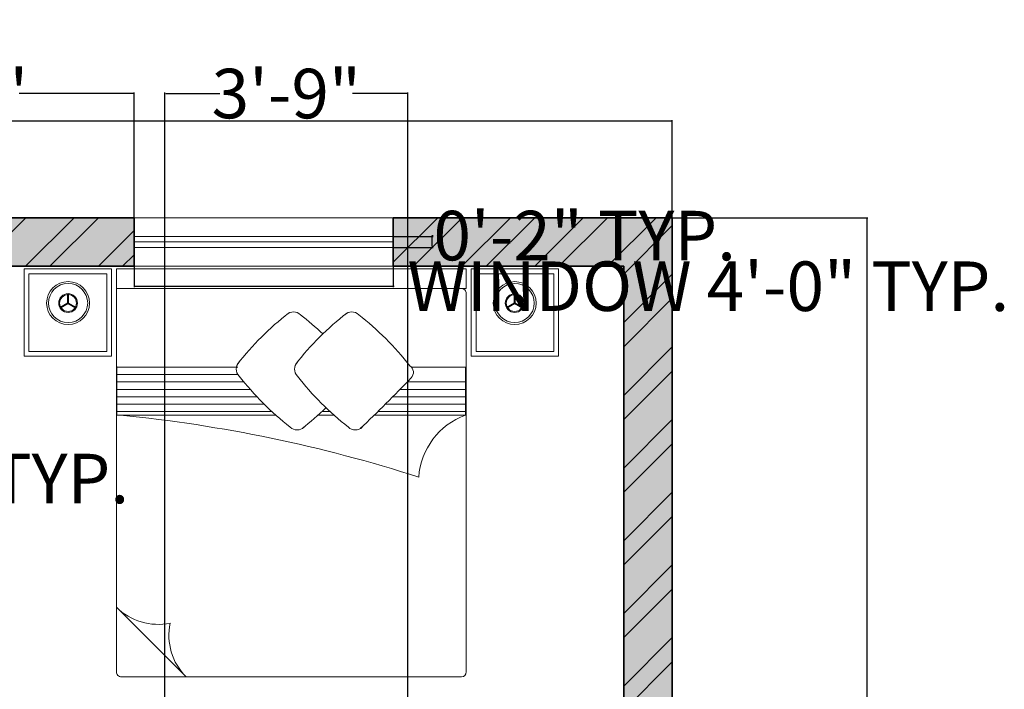
# Model space of a CAD drawing. Units: inches. Extents: x 1086 to 1540, y 3343 to 3848.
# Tile 8 of 8: x 1350 to 1532, y 3724 to 3848. Entities that reach past the tile are written whole.
import ezdxf

# ---------------------------------------------------------------- set-up
doc = ezdxf.new("R2010")
doc.units = ezdxf.units.IN
for name, color, linetype, lineweight in [('00 FURNITURE', 15, 'Continuous', 15), ('A-ANNO-DIMS', 2, 'Continuous', 13), ('A-WALL-PATT', 252, 'Continuous', 9), ('WALL', 7, 'Continuous', 35), ('WINDOW', 160, 'Continuous', 15)]:
    doc.layers.add(name, color=color, linetype=linetype, lineweight=lineweight)
doc.styles.get("Standard").update_dxf_attribs({"font": 'arial.ttf'})
doc.dimstyles.get("Standard").update_dxf_attribs({"dimtxt": 9.18, "dimasz": 0.18, "dimexe": 0.18, "dimexo": 0.0625, "dimgap": 0.09, "dimtad": 0, "dimtih": 1, "dimtoh": 1, "dimdec": 1, "dimzin": 0, "dimdsep": 46, "dimlunit": 3, "dimtxsty": 'Standard', "dimcen": 0.09, "dimadec": 0, "dimazin": 0, "dimtfac": 1, "dimtdec": 1, "dimtofl": 0, "dimtmove": 0, "dimatfit": 3, "dimfxl": 1, "dimtolj": 1, "dimtzin": 0, "dimarcsym": 0})

# ---------------------------------------------------------------- blocks, each defined once
blk = doc.blocks.new('RGWTG')
at = {"layer": '00 FURNITURE'}
for p, q in [((578.23, 3473.51), (577.36, 3475.01)), ((578.36, 3473.58), (577.49, 3475.09)), ((578.23, 3473.58), (577.36, 3472.08)), ((578.36, 3473.51), (577.49, 3472)), ((578.29, 3473.62), (580.03, 3473.62)), ((578.29, 3473.47), (580.03, 3473.47)), ((521.93, 3464.58), (509.03, 3451.68)), ((509.03, 3422.63), (509.03, 3463.68)), ((509.93, 3464.58), (566.4, 3464.58)), ((557.53, 3463.84), (557.53, 3464.49)), ((557.53, 3464.49), (566.4, 3464.49)), ((558.2, 3464.49), (558.2, 3435.82)), ((559.57, 3464.49), (559.57, 3437.25)), ((560.94, 3464.49), (560.94, 3438.58)), ((562.3, 3464.49), (562.3, 3439.83)), ((563.67, 3464.49), (563.67, 3440.99)), ((565.04, 3464.49), (565.04, 3442.08)), ((566.4, 3464.58), (580.98, 3464.58)), ((566.4, 3464.49), (566.4, 3442.08)), ((566.4, 3464.49), (566.4, 3463.84)), ((580.98, 3464.58), (580.98, 3416.72)), ((558.2, 3426.48), (558.2, 3425.04)), ((509.03, 3400.68), (509.03, 3422.63)), ((558.2, 3416.13), (558.2, 3399.95)), ((580.98, 3416.72), (580.98, 3400.68)), ((559.57, 3414.75), (559.57, 3399.95)), ((560.94, 3413.39), (560.94, 3399.95)), ((562.3, 3412.04), (562.3, 3399.95)), ((563.67, 3410.72), (563.67, 3399.95)), ((580.08, 3399.78), (509.93, 3399.78)), ((557.53, 3399.95), (557.53, 3400.6)), ((566.4, 3399.95), (557.53, 3399.95)), ((566.4, 3400.6), (566.4, 3399.95)), ((578.23, 3390.78), (577.36, 3392.29)), ((578.36, 3390.86), (577.49, 3392.36)), ((578.23, 3390.86), (577.36, 3389.36)), ((578.36, 3390.78), (577.49, 3389.28)), ((578.29, 3390.9), (580.03, 3390.9)), ((578.29, 3390.74), (580.03, 3390.74))]:
    blk.add_line(p, q, dxfattribs=at)
for points in [[(568.43, 3465.48), (584.63, 3465.48), (584.63, 3481.68), (568.43, 3481.68)], [(569.33, 3466.38), (583.73, 3466.38), (583.73, 3480.78), (569.33, 3480.78)], [(580.98, 3399.78), (584.63, 3399.78), (584.63, 3464.58), (580.98, 3464.58)], [(568.43, 3398.88), (584.63, 3398.88), (584.63, 3382.68), (568.43, 3382.68)], [(569.33, 3397.98), (583.73, 3397.98), (583.73, 3383.58), (569.33, 3383.58)]]:
    blk.add_lwpolyline(points, close=True, dxfattribs=at)
for points in [[(566.52, 3464.49), (557.53, 3464.49), (557.53, 3435.08)], [(557.53, 3427.21), (557.53, 3424.3)], [(557.53, 3416.82), (557.53, 3399.95), (566.4, 3399.95), (566.4, 3409.94)]]:
    blk.add_lwpolyline(points, dxfattribs=at)
for centre, radius in [((578.29, 3473.54), 3.97), ((578.29, 3473.54), 3.63), ((578.29, 3473.54), 1.74), ((578.29, 3473.54), 1.56), ((578.29, 3390.82), 3.97), ((578.29, 3390.82), 3.63), ((578.29, 3390.82), 1.74), ((578.29, 3390.82), 1.56)]:
    blk.add_circle(centre, radius, dxfattribs=at)
for centre, radius, start, end in [((509.93, 3463.68), 0.9, 90, 180), ((529.65, 3456.88), 10.9, 135.0361, 191.9278), ((290.56, 3490.52), 268.3, 342.2214, 354.2925), ((516.73, 3443.97), 10.9, 78.0722, 134.9639), ((598.15, 3399.01), 54.32, 127.931, 142.069), ((566.05, 3440.57), 1.82, 45, 135), ((533.58, 3399.31), 54.32, 37.931, 52.069), ((556.59, 3431.11), 1.82, 135, 225), ((574.84, 3431.77), 1.82, 315, 45), ((598.15, 3388.23), 54.32, 127.931, 142.069), ((566.05, 3429.78), 1.82, 45, 135), ((533.58, 3388.53), 54.32, 37.931, 52.069), ((533.28, 3463.88), 54.32, 316.32, 322.069), ((597.87, 3463.6), 54.32, 217.931, 224.141), ((556.59, 3420.33), 1.82, 135, 225), ((574.84, 3420.99), 1.82, 315, 45), ((765.33, 3619.75), 290.45, 223.6069, 226.2326), ((533.28, 3453.1), 54.32, 307.931, 322.069), ((545.02, 3395.29), 13.35, 20.4224, 85.5825), ((565.44, 3411.05), 1.47, 225.9674, 326.8337), ((509.93, 3400.68), 0.9, 180, 270), ((580.08, 3400.68), 0.9, 270, 0)]:
    blk.add_arc(centre, radius, start, end, dxfattribs=at)
blk = doc.blocks.new('*D12')
at = {"layer": 'A-ANNO-DIMS', "color": 0, "lineweight": -2, "transparency": 16777216}
for p, q in [((1194.74, 3811.63), (1194.74, 3829.64)), ((1194.92, 3829.46), (1324.78, 3829.46)), ((1470.56, 3829.46), (1340.7, 3829.46)), ((1470.74, 3811.63), (1470.74, 3829.64))]:
    blk.add_line(p, q, dxfattribs=at)
at = {"layer": 'A-ANNO-DIMS', "color": 0, "transparency": 16777216}
for points in [[(1194.92, 3829.49), (1194.92, 3829.43), (1194.74, 3829.46)], [(1470.56, 3829.49), (1470.56, 3829.43), (1470.74, 3829.46)]]:
    blk.add_solid(points, dxfattribs=at)
at = {"layer": 'Defpoints', "color": 0, "transparency": 16777216}
for p in [(1470.74, 3829.46), (1194.74, 3811.57), (1470.74, 3811.57)]:
    blk.add_point(p, dxfattribs=at)
at = {"layer": 'A-ANNO-DIMS', "color": 0, "transparency": 16777216, "insert": (1332.74, 3829.46), "char_height": 9.18, "attachment_point": 5}
blk.add_mtext("\\A1;23'", dxfattribs=at)
blk = doc.blocks.new('*D13')
at = {"layer": 'A-ANNO-DIMS', "color": 0, "lineweight": -2, "transparency": 16777216}
for p, q in [((1470.8, 3811.57), (1506.93, 3811.57)), ((1506.75, 3811.39), (1506.75, 3600.35)), ((1506.75, 3379.75), (1506.75, 3590.79)), ((1470.8, 3379.57), (1506.93, 3379.57))]:
    blk.add_line(p, q, dxfattribs=at)
at = {"layer": 'A-ANNO-DIMS', "color": 0, "transparency": 16777216}
for points in [[(1506.72, 3811.39), (1506.78, 3811.39), (1506.75, 3811.57)], [(1506.72, 3379.75), (1506.78, 3379.75), (1506.75, 3379.57)]]:
    blk.add_solid(points, dxfattribs=at)
at = {"layer": 'Defpoints', "color": 0, "transparency": 16777216}
for p in [(1470.74, 3811.57), (1470.74, 3379.57), (1506.75, 3379.57)]:
    blk.add_point(p, dxfattribs=at)
at = {"layer": 'A-ANNO-DIMS', "color": 0, "transparency": 16777216, "insert": (1506.75, 3595.57), "char_height": 9.18, "attachment_point": 5}
blk.add_mtext("\\A1;36'", dxfattribs=at)
blk = doc.blocks.new('WIN-GLAZING-48IN')
for p, q in [((48, 1), (0, 1)), ((48, 0), (0, 0)), ((48, -1), (0, -1))]:
    blk.add_line(p, q)
blk = doc.blocks.new('*D22')
at = {"layer": 'A-ANNO-DIMS', "color": 0, "lineweight": -2, "transparency": 16777216}
for p, q in [((1316.51, 3801.03), (1331.48, 3801.03)), ((1331.3, 3800.85), (1331.3, 3768.07)), ((1331.3, 3725.61), (1331.3, 3758.39)), ((1316.51, 3725.43), (1331.48, 3725.43))]:
    blk.add_line(p, q, dxfattribs=at)
at = {"layer": 'A-ANNO-DIMS', "color": 0, "transparency": 16777216}
for points in [[(1331.27, 3800.85), (1331.33, 3800.85), (1331.3, 3801.03)], [(1331.27, 3725.61), (1331.33, 3725.61), (1331.3, 3725.43)]]:
    blk.add_solid(points, dxfattribs=at)
at = {"layer": 'Defpoints', "color": 0, "transparency": 16777216}
for p in [(1316.45, 3801.03), (1331.3, 3801.03), (1316.45, 3725.43)]:
    blk.add_point(p, dxfattribs=at)
at = {"layer": 'A-ANNO-DIMS', "color": 0, "transparency": 16777216, "insert": (1331.3, 3763.23), "char_height": 9.18, "attachment_point": 5}
blk.add_mtext('\\A1;6\'-3 1/2" TYP.', dxfattribs=at)
blk = doc.blocks.new('*D23')
at = {"layer": 'A-ANNO-DIMS', "color": 0, "lineweight": -2, "transparency": 16777216}
for p, q in [((1371.06, 3806.01), (1371.06, 3798.69)), ((1419.06, 3806.01), (1419.06, 3798.69)), ((1371.24, 3798.87), (1418.88, 3798.87)), ((1419.06, 3798.87), (1419.24, 3798.87))]:
    blk.add_line(p, q, dxfattribs=at)
at = {"layer": 'A-ANNO-DIMS', "color": 0, "transparency": 16777216}
for points in [[(1371.24, 3798.9), (1371.24, 3798.84), (1371.06, 3798.87)], [(1418.88, 3798.9), (1418.88, 3798.84), (1419.06, 3798.87)]]:
    blk.add_solid(points, dxfattribs=at)
at = {"layer": 'Defpoints', "color": 0, "transparency": 16777216}
for p in [(1371.06, 3806.07), (1419.06, 3806.07), (1419.06, 3798.87)]:
    blk.add_point(p, dxfattribs=at)
at = {"layer": 'A-ANNO-DIMS', "color": 0, "transparency": 16777216, "insert": (1477.41, 3798.87), "char_height": 9.18, "attachment_point": 5}
blk.add_mtext('\\A1;WINDOW 4\'-0" TYP.', dxfattribs=at)
blk = doc.blocks.new('*D24')
at = {"layer": 'A-ANNO-DIMS', "color": 0, "lineweight": -2, "transparency": 16777216}
for p, q in [((1419.12, 3808.07), (1426.44, 3808.07)), ((1426.26, 3808.07), (1426.26, 3808.25)), ((1426.26, 3808.25), (1426.44, 3808.25)), ((1426.26, 3806.25), (1426.26, 3807.89)), ((1419.12, 3806.07), (1426.44, 3806.07))]:
    blk.add_line(p, q, dxfattribs=at)
at = {"layer": 'A-ANNO-DIMS', "color": 0, "transparency": 16777216}
for points in [[(1426.23, 3807.89), (1426.29, 3807.89), (1426.26, 3808.07)], [(1426.23, 3806.25), (1426.29, 3806.25), (1426.26, 3806.07)]]:
    blk.add_solid(points, dxfattribs=at)
at = {"layer": 'Defpoints', "color": 0, "transparency": 16777216}
for p in [(1419.06, 3808.07), (1426.26, 3808.07), (1419.06, 3806.07)]:
    blk.add_point(p, dxfattribs=at)
at = {"layer": 'A-ANNO-DIMS', "color": 0, "transparency": 16777216, "insert": (1454.51, 3808.25), "char_height": 9.18, "attachment_point": 5}
blk.add_mtext('\\A1;0\'-2" TYP.', dxfattribs=at)
blk = doc.blocks.new('*D48')
at = {"layer": 'A-ANNO-DIMS', "color": 0, "lineweight": -2, "transparency": 16777216}
for p, q in [((1282.55, 3811.63), (1282.55, 3834.75)), ((1282.73, 3834.57), (1303.86, 3834.57)), ((1370.88, 3834.57), (1349.75, 3834.57)), ((1371.06, 3811.63), (1371.06, 3834.75))]:
    blk.add_line(p, q, dxfattribs=at)
at = {"layer": 'A-ANNO-DIMS', "color": 0, "transparency": 16777216}
for points in [[(1282.73, 3834.6), (1282.73, 3834.54), (1282.55, 3834.57)], [(1370.88, 3834.6), (1370.88, 3834.54), (1371.06, 3834.57)]]:
    blk.add_solid(points, dxfattribs=at)
at = {"layer": 'Defpoints', "color": 0, "transparency": 16777216}
for p in [(1371.06, 3834.57), (1282.55, 3811.57), (1371.06, 3811.57)]:
    blk.add_point(p, dxfattribs=at)
at = {"layer": 'A-ANNO-DIMS', "color": 0, "transparency": 16777216, "insert": (1326.8, 3834.57), "char_height": 9.18, "attachment_point": 5}
blk.add_mtext('\\A1;7\'-4 1/2"', dxfattribs=at)
blk = doc.blocks.new('*D70')
at = {"layer": 'A-ANNO-DIMS', "color": 0, "lineweight": -2, "transparency": 16777216}
for p, q in [((1376.74, 3634.63), (1376.74, 3834.75)), ((1376.92, 3834.57), (1386.95, 3834.57)), ((1421.56, 3834.57), (1411.53, 3834.57)), ((1421.74, 3634.63), (1421.74, 3834.75))]:
    blk.add_line(p, q, dxfattribs=at)
at = {"layer": 'A-ANNO-DIMS', "color": 0, "transparency": 16777216}
for points in [[(1376.92, 3834.6), (1376.92, 3834.54), (1376.74, 3834.57)], [(1421.56, 3834.6), (1421.56, 3834.54), (1421.74, 3834.57)]]:
    blk.add_solid(points, dxfattribs=at)
at = {"layer": 'Defpoints', "color": 0, "transparency": 16777216}
for p in [(1421.74, 3834.57), (1376.74, 3634.57), (1421.74, 3634.57)]:
    blk.add_point(p, dxfattribs=at)
at = {"layer": 'A-ANNO-DIMS', "color": 0, "transparency": 16777216, "insert": (1399.24, 3834.57), "char_height": 9.18, "attachment_point": 5}
blk.add_mtext('\\A1;3\'-9"', dxfattribs=at)

msp = doc.modelspace()

# ---------------------------------------------------------------- hatches: boundary and pattern name
at = {"layer": 'A-WALL-PATT'}
h = msp.add_hatch(dxfattribs=at)
h.set_pattern_fill('ANSI32', color=256)
h.paths.add_polyline_path([(1234.55, 3811.57), (1234.55, 3811.57), (1194.74, 3811.57), (1194.74, 3622.57), (1203.74, 3622.57), (1203.74, 3634.57), (1218.33, 3634.57), (1218.33, 3638.57), (1203.74, 3638.57), (1203.74, 3802.57), (1234.55, 3802.57)])
h.paths.add_polyline_path([(1371.06, 3811.57), (1371.06, 3811.57), (1282.55, 3811.57), (1282.55, 3802.57), (1331.74, 3802.57), (1331.74, 3634.57), (1335.74, 3634.57), (1335.74, 3639.57), (1335.74, 3802.57), (1371.06, 3802.57)])
h.paths.add_polyline_path([(1470.74, 3811.57), (1419.06, 3811.57), (1419.06, 3802.57), (1461.74, 3802.57), (1461.74, 3638.57), (1461.74, 3548.57), (1425.74, 3548.57), (1425.74, 3582.21), (1421.74, 3582.21), (1421.74, 3548.57), (1376.74, 3548.57), (1376.74, 3602.57), (1373.71, 3602.57), (1372.74, 3602.57), (1372.74, 3544.57), (1461.74, 3544.57), (1461.74, 3379.57), (1470.74, 3379.57)])
h.paths.add_polyline_path([(1203.74, 3582.57), (1295.74, 3582.57), (1295.74, 3586.57), (1203.74, 3586.57), (1203.74, 3598.57), (1194.74, 3598.57), (1194.74, 3379.57), (1326.74, 3379.57), (1326.74, 3388.57), (1322.74, 3388.57), (1203.74, 3388.57), (1203.74, 3451.57), (1234.74, 3451.57), (1234.74, 3455.57), (1203.74, 3455.57), (1203.74, 3479.57), (1203.74, 3544.57), (1227.74, 3544.57), (1253.74, 3544.57), (1253.74, 3548.57), (1203.74, 3548.57)])
h.paths.add_polyline_path([(1461.74, 3638.57), (1371.74, 3638.57), (1371.74, 3634.57), (1372.74, 3634.57), (1372.74, 3632.57), (1376.74, 3632.57), (1376.74, 3634.57), (1421.74, 3634.57), (1421.74, 3606.21), (1425.74, 3606.21), (1425.74, 3634.57), (1461.74, 3634.57)])
h.paths.add_polyline_path([(1295.74, 3638.57), (1266.33, 3638.57), (1266.33, 3634.57), (1292.74, 3634.57), (1295.74, 3634.57)])
h.paths.add_polyline_path([(1322.74, 3548.57), (1318.74, 3548.57), (1318.74, 3455.57), (1282.74, 3455.57), (1282.74, 3451.57), (1318.74, 3451.57), (1318.74, 3420.07), (1322.74, 3420.07)], flags=17)
at = {"layer": 'A-WALL-PATT', "transparency": 33554559}
h = msp.add_hatch(color=256, dxfattribs=at)
h.dxf.hatch_style = 1
h.paths.add_polyline_path([(1234.55, 3811.57), (1234.55, 3811.57), (1194.74, 3811.57), (1194.74, 3622.57), (1203.74, 3622.57), (1203.74, 3634.57), (1218.33, 3634.57), (1218.33, 3638.57), (1203.74, 3638.57), (1203.74, 3802.57), (1234.55, 3802.57)])
h.paths.add_polyline_path([(1371.06, 3811.57), (1371.06, 3811.57), (1282.55, 3811.57), (1282.55, 3802.57), (1331.74, 3802.57), (1331.74, 3634.57), (1335.74, 3634.57), (1335.74, 3639.57), (1335.74, 3802.57), (1371.06, 3802.57)])
h.paths.add_polyline_path([(1470.74, 3811.57), (1419.06, 3811.57), (1419.06, 3802.57), (1461.74, 3802.57), (1461.74, 3638.57), (1461.74, 3548.57), (1425.74, 3548.57), (1425.74, 3582.21), (1421.74, 3582.21), (1421.74, 3548.57), (1376.74, 3548.57), (1376.74, 3602.57), (1372.74, 3602.57), (1372.74, 3544.57), (1461.74, 3544.57), (1461.74, 3379.57), (1470.74, 3379.57)])
h.paths.add_polyline_path([(1203.74, 3544.57), (1227.74, 3544.57), (1253.74, 3544.57), (1253.74, 3548.57), (1203.74, 3548.57), (1203.74, 3582.57), (1295.74, 3582.57), (1295.74, 3586.57), (1203.74, 3586.57), (1203.74, 3598.57), (1194.74, 3598.57), (1194.74, 3379.57), (1326.74, 3379.57), (1326.74, 3388.57), (1322.74, 3388.57), (1203.74, 3388.57), (1203.74, 3451.57), (1234.74, 3451.57), (1234.74, 3455.57), (1203.74, 3455.57)])
h.paths.add_polyline_path([(1413.74, 3388.57), (1413.74, 3388.57), (1374.74, 3388.57), (1374.74, 3383.18), (1374.74, 3383.18), (1374.74, 3379.57), (1413.74, 3379.57)], flags=17)
h.paths.add_polyline_path([(1322.74, 3548.57), (1318.74, 3548.57), (1318.74, 3455.57), (1282.74, 3455.57), (1282.74, 3451.57), (1318.74, 3451.57), (1318.74, 3420.07), (1322.74, 3420.07)], flags=17)
h.paths.add_polyline_path([(1295.74, 3638.57), (1266.33, 3638.57), (1266.33, 3634.57), (1292.74, 3634.57), (1295.74, 3634.57)])
h.paths.add_polyline_path([(1461.74, 3638.57), (1371.74, 3638.57), (1371.74, 3634.57), (1372.74, 3634.57), (1372.74, 3632.57), (1376.74, 3632.57), (1376.74, 3634.57), (1421.74, 3634.57), (1421.74, 3606.21), (1425.74, 3606.21), (1425.74, 3634.57), (1461.74, 3634.57)])

# ---------------------------------------------------------------- linework, layer by layer
at = {"layer": 'WALL'}
for p, q in [((1282.55, 3811.57), (1371.06, 3811.57)), ((1371.06, 3802.57), (1371.06, 3811.57)), ((1419.06, 3802.57), (1419.06, 3811.57)), ((1419.06, 3811.57), (1470.74, 3811.57)), ((1470.74, 3811.57), (1470.74, 3379.57)), ((1335.74, 3802.57), (1371.06, 3802.57)), ((1419.06, 3802.57), (1461.74, 3802.57)), ((1461.74, 3802.57), (1461.74, 3638.57))]:
    msp.add_line(p, q, dxfattribs=at)
at = {"layer": 'WINDOW'}
for p, q in [((1419.06, 3811.57), (1371.06, 3811.57)), ((1371.06, 3802.57), (1419.06, 3802.57))]:
    msp.add_line(p, q, dxfattribs=at)

# ---------------------------------------------------------------- block references
at = {"layer": '00 FURNITURE', "rotation": 89.99999999999999}
msp.add_blockref('RGWTG', (4832.36, 3217.46), dxfattribs=at)
at = {"layer": 'WINDOW'}
msp.add_blockref('WIN-GLAZING-48IN', (1371.06, 3807.07), dxfattribs=at)

# ---------------------------------------------------------------- dimensions: what is measured, and where the dimension line sits
at = {"layer": 'A-ANNO-DIMS'}
for base, p1, p2, override, picture, middle in [((1371.06, 3834.57), (1282.55, 3811.57), (1371.06, 3811.57), {"dimdec": 1, "dimlfac": 1, "dimrnd": 0, "dimzin": 1, "dimdsep": 46, "dimlunit": 4, "dimfrac": 2}, '*D48', (1326.8, 3834.57)), ((1421.74, 3834.57), (1376.74, 3634.57), (1421.74, 3634.57), {"dimdec": 1, "dimlfac": 1, "dimrnd": 0, "dimzin": 1, "dimdsep": 46, "dimlunit": 4, "dimfrac": 2}, '*D70', (1399.24, 3834.57)), ((1470.74, 3829.46), (1194.74, 3811.57), (1470.74, 3811.57), {"dimclrd": 0, "dimclre": 0, "dimclrt": 0}, '*D12', (1332.74, 3829.46))]:
    dim = msp.add_linear_dim(base=base, p1=p1, p2=p2, dimstyle='Standard', override=override, dxfattribs=at)
    dim.commit()
    dim.dimension.update_dxf_attribs({"geometry": picture, "text_midpoint": middle})
for base, p1, p2, picture, middle in [((1426.26, 3808.07), (1419.06, 3806.07), (1419.06, 3808.07), '*D24', (1454.51, 3808.25)), ((1331.3, 3801.03), (1316.45, 3725.43), (1316.45, 3801.03), '*D22', (1331.3, 3763.23))]:
    dim = msp.add_linear_dim(base=base, p1=p1, p2=p2, angle=90, text='<> TYP.', dimstyle='Standard', override={"dimdec": 1, "dimlfac": 1, "dimrnd": 0, "dimzin": 1, "dimdsep": 46, "dimlunit": 4, "dimfrac": 2}, dxfattribs=at)
    dim.commit()
    dim.dimension.update_dxf_attribs({"geometry": picture, "text_midpoint": middle})
dim = msp.add_linear_dim(base=(1419.06, 3798.87), p1=(1371.06, 3806.07), p2=(1419.06, 3806.07), text='WINDOW <> TYP.', dimstyle='Standard', override={"dimdec": 1, "dimlfac": 1, "dimrnd": 0, "dimzin": 1, "dimdsep": 46, "dimlunit": 4, "dimfrac": 2}, dxfattribs=at)
dim.commit()
dim.dimension.update_dxf_attribs({"geometry": '*D23', "text_midpoint": (1477.41, 3798.87)})
dim = msp.add_linear_dim(base=(1506.75, 3379.57), p1=(1470.74, 3811.57), p2=(1470.74, 3379.57), angle=90, dimstyle='Standard', override={"dimclrd": 0, "dimclre": 0, "dimclrt": 0}, dxfattribs=at)
dim.commit()
dim.dimension.update_dxf_attribs({"geometry": '*D13', "text_midpoint": (1506.75, 3595.57)})

doc.saveas('drawing.dxf')
